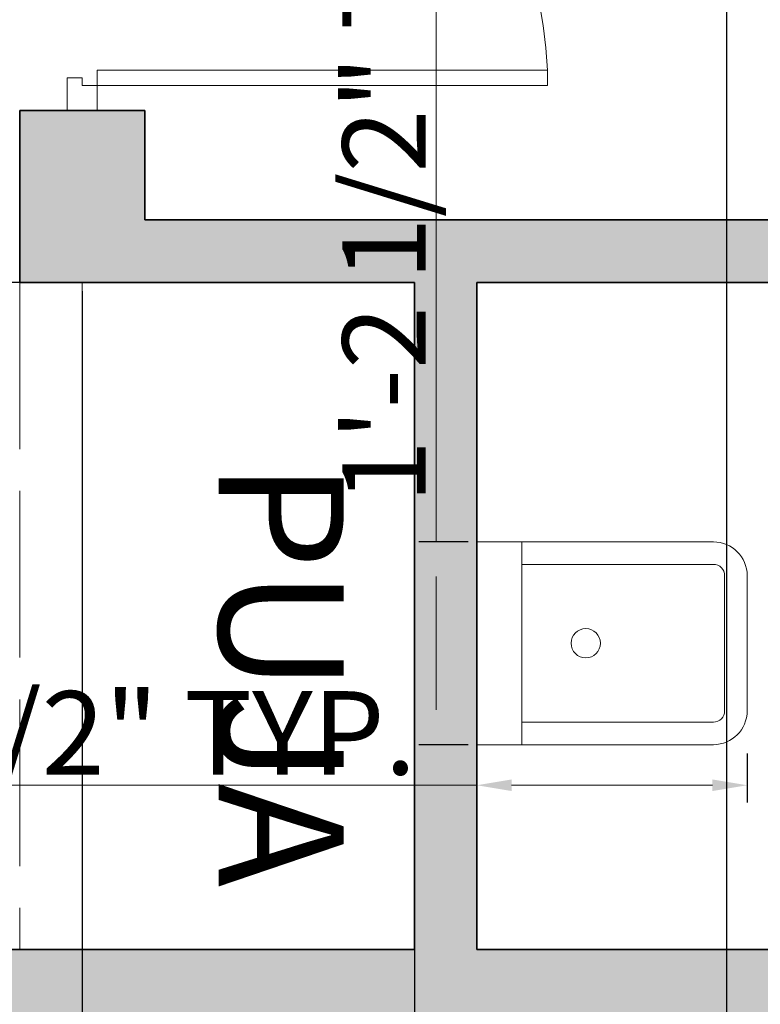
# Model space of a CAD drawing. Units: inches. Extents: x 2696 to 3240, y 1564 to 2310.
# Tile 66 of 76: x 3074 to 3127, y 2071 to 2142. Entities that reach past the tile are written whole.
import ezdxf

# ---------------------------------------------------------------- set-up
doc = ezdxf.new("R2010")
doc.units = ezdxf.units.IN
doc.linetypes.add('ACAD_ISO02W100', pattern=[15, 12, -3])
for name, color, linetype, lineweight in [('A-ANNO-DIMS', 3, 'Continuous', 18), ('A-AREA-IDEN', 7, 'Continuous', 18), ('A-DOOR', 4, 'Continuous', 18), ('A-FLOR-FIXT', 8, 'Continuous', 18), ('A-FURN', 251, 'Continuous', 13), ('A-WALL', 7, 'Continuous', 35), ('A-WALL-OVHD', 7, 'ACAD_ISO02W100', 18), ('A-WALL-PATT', 9, 'Continuous', 13)]:
    doc.layers.add(name, color=color, linetype=linetype, lineweight=lineweight)
doc.styles.add('TIMES NEW', font='times.ttf')
doc.styles.add('YQ_DIM', font='SUPEROS.SHX', dxfattribs={"width": 0.8, "bigfont": 'HZDX.SHX'})
doc.dimstyles.new('Siddhuu', dxfattribs={"dimtxt": 6, "dimasz": 2.5, "dimexe": 1.25, "dimexo": 0.625, "dimtad": 1, "dimdec": 1, "dimlunit": 4, "dimtxsty": 'TIMES NEW', "dimcen": 2.5, "dimclrd": 256, "dimclre": 1, "dimclrt": 7, "dimadec": 0, "dimazin": 0, "dimtfac": 1, "dimtdec": 1, "dimtmove": 0, "dimatfit": 3, "dimfxl": 1, "dimtolj": 1, "dimlwd": -1, "dimarcsym": 0})

# ---------------------------------------------------------------- blocks, each defined once
blk = doc.blocks.new('DR_D01')
for p, q in [((-0.45, 0.93), (-0.42, 0.93)), ((-0.45, 0.03), (-0.45, 0.93)), ((-0.42, 0.03), (-0.42, 0.93)), ((-0.5, 0.03), (-0.42, 0.03)), ((-0.5, 0.03), (-0.5, -0.03)), ((-0.45, 0.03), (-0.45, 0)), ((0.45, 0.03), (0.45, 0)), ((0.5, 0.03), (0.45, 0.03)), ((0.5, -0.03), (0.5, 0.03)), ((-0.45, 0), (-0.435, 0)), ((-0.435, 0), (-0.435, -0.03)), ((0.435, 0), (0.435, -0.03)), ((0.45, 0), (0.435, 0)), ((-0.435, -0.03), (-0.5, -0.03)), ((0.435, -0.03), (0.5, -0.03))]:
    blk.add_line(p, q)
blk.add_arc((-0.4602, 0.0206), 0.9103, 0.5915, 87.4664)
blk = doc.blocks.new('WC')
at = {"layer": 'A-FURN'}
for p, q in [((0, 14.59), (-17.022, 14.59)), ((-3.242, 14.59), (-3.242, 0)), ((-3.242, 12.969), (-17.022, 12.969)), ((-19.454, 2.432), (-19.454, 12.159)), ((-17.833, 2.432), (-17.833, 12.159)), ((-3.242, 1.621), (-17.022, 1.621)), ((0, 0), (-17.022, 0))]:
    blk.add_line(p, q, dxfattribs=at)
blk.add_circle((-7.836, 7.295), 1.051, dxfattribs=at)
for centre, radius, start, end in [((-17.022, 12.159), 2.432, 90, 180), ((-17.022, 12.159), 0.811, 90, 180), ((-17.022, 2.432), 2.432, 180, 270), ((-17.022, 2.432), 0.811, 180, 270)]:
    blk.add_arc(centre, radius, start, end, dxfattribs=at)
blk = doc.blocks.new('*D38')
at = {"layer": 'A-ANNO-DIMS', "color": 1, "lineweight": -2, "transparency": 16777216}
for p, q in [((3106.611, 2088.816), (3106.611, 2085.273)), ((3126.065, 2088.816), (3126.065, 2085.273))]:
    blk.add_line(p, q, dxfattribs=at)
at = {"layer": 'A-ANNO-DIMS', "transparency": 16777216}
for p, q in [((3106.611, 2086.523), (3035.395, 2086.523)), ((3123.565, 2086.523), (3109.111, 2086.523))]:
    blk.add_line(p, q, dxfattribs=at)
for points in [[(3109.111, 2086.94), (3109.111, 2086.107), (3106.611, 2086.523)], [(3123.565, 2086.94), (3123.565, 2086.107), (3126.065, 2086.523)]]:
    blk.add_solid(points, dxfattribs=at)
at = {"layer": 'Defpoints', "color": 0, "transparency": 16777216}
for p in [(3106.611, 2089.441), (3126.065, 2089.441), (3106.611, 2086.523)]:
    blk.add_point(p, dxfattribs=at)
at = {"layer": 'A-ANNO-DIMS', "color": 7, "transparency": 16777216, "insert": (3069.753, 2090.291), "char_height": 6, "attachment_point": 5, "style": 'TIMES NEW'}
blk.add_mtext('\\A1;WC 1\'-7 1/2" TYP.', dxfattribs=at)
blk = doc.blocks.new('*D39')
at = {"layer": 'A-ANNO-DIMS', "transparency": 16777216}
for p, q in [((3103.693, 2104.032), (3103.693, 2157.841)), ((3103.693, 2091.941), (3103.693, 2101.532))]:
    blk.add_line(p, q, dxfattribs=at)
at = {"layer": 'A-ANNO-DIMS', "color": 1, "lineweight": -2, "transparency": 16777216}
for p, q in [((3105.986, 2104.032), (3102.443, 2104.032)), ((3105.986, 2089.441), (3102.443, 2089.441))]:
    blk.add_line(p, q, dxfattribs=at)
at = {"layer": 'A-ANNO-DIMS', "transparency": 16777216}
for points in [[(3103.277, 2101.532), (3104.11, 2101.532), (3103.693, 2104.032)], [(3103.277, 2091.941), (3104.11, 2091.941), (3103.693, 2089.441)]]:
    blk.add_solid(points, dxfattribs=at)
at = {"layer": 'Defpoints', "color": 0, "transparency": 16777216}
for p in [(3103.693, 2104.032), (3106.611, 2104.032), (3106.611, 2089.441)]:
    blk.add_point(p, dxfattribs=at)
at = {"layer": 'A-ANNO-DIMS', "color": 7, "transparency": 16777216, "insert": (3099.932, 2132.186), "char_height": 6, "attachment_point": 5, "rotation": 90, "style": 'TIMES NEW'}
blk.add_mtext('\\A1;1\'-2 1/2" TYP.', dxfattribs=at)
blk = doc.blocks.new('*D54')
at = {"layer": 'A-ANNO-DIMS', "color": 1, "lineweight": -2, "transparency": 16777216}
for p, q in [((3124.611, 1893.826), (3124.611, 2298.451)), ((3136.611, 1893.826), (3136.611, 2298.451))]:
    blk.add_line(p, q, dxfattribs=at)
at = {"layer": 'A-ANNO-DIMS', "transparency": 16777216}
for p, q in [((3127.111, 2297.201), (3134.111, 2297.201)), ((3136.611, 2297.201), (3155.757, 2297.201))]:
    blk.add_line(p, q, dxfattribs=at)
for points in [[(3127.111, 2297.618), (3127.111, 2296.784), (3124.611, 2297.201)], [(3134.111, 2297.618), (3134.111, 2296.784), (3136.611, 2297.201)]]:
    blk.add_solid(points, dxfattribs=at)
at = {"layer": 'Defpoints', "color": 0, "transparency": 16777216}
for p in [(3136.611, 2297.201), (3124.611, 1893.201), (3136.611, 1893.201)]:
    blk.add_point(p, dxfattribs=at)
at = {"layer": 'A-ANNO-DIMS', "color": 7, "transparency": 16777216, "insert": (3147.434, 2300.878), "char_height": 6, "attachment_point": 5, "style": 'TIMES NEW'}
blk.add_mtext('\\A1;1\'-0"', dxfattribs=at)
blk = doc.blocks.new('*D65')
at = {"layer": 'A-ANNO-DIMS', "color": 1, "lineweight": -2, "transparency": 16777216}
for p, q in [((3078.209, 2122.076), (3078.209, 1568.951)), ((3102.111, 2122.076), (3102.111, 1568.951))]:
    blk.add_line(p, q, dxfattribs=at)
at = {"layer": 'A-ANNO-DIMS', "transparency": 16777216}
blk.add_line((3080.709, 1570.201), (3099.611, 1570.201), dxfattribs=at)
for points in [[(3080.709, 1570.618), (3080.709, 1569.784), (3078.209, 1570.201)], [(3099.611, 1570.618), (3099.611, 1569.784), (3102.111, 1570.201)]]:
    blk.add_solid(points, dxfattribs=at)
at = {"layer": 'Defpoints', "color": 0, "transparency": 16777216}
for p in [(3078.209, 2122.701), (3102.111, 2122.701), (3102.111, 1570.201)]:
    blk.add_point(p, dxfattribs=at)
at = {"layer": 'A-ANNO-DIMS', "color": 7, "transparency": 16777216, "insert": (3090.16, 1573.878), "char_height": 6, "attachment_point": 5, "style": 'TIMES NEW'}
blk.add_mtext('\\A1;2\'-0"', dxfattribs=at)
blk = doc.blocks.new('*D66')
at = {"layer": 'A-ANNO-DIMS', "color": 1, "lineweight": -2, "transparency": 16777216}
for p, q in [((3077.584, 2122.701), (2709.361, 2122.701)), ((3077.584, 2074.701), (2709.361, 2074.701))]:
    blk.add_line(p, q, dxfattribs=at)
at = {"layer": 'A-ANNO-DIMS', "transparency": 16777216}
blk.add_line((2710.611, 2077.201), (2710.611, 2120.201), dxfattribs=at)
for points in [[(2710.195, 2120.201), (2711.028, 2120.201), (2710.611, 2122.701)], [(2710.195, 2077.201), (2711.028, 2077.201), (2710.611, 2074.701)]]:
    blk.add_solid(points, dxfattribs=at)
at = {"layer": 'Defpoints', "color": 0, "transparency": 16777216}
for p in [(2710.611, 2122.701), (3078.209, 2122.701), (3078.209, 2074.701)]:
    blk.add_point(p, dxfattribs=at)
at = {"layer": 'A-ANNO-DIMS', "color": 7, "transparency": 16777216, "insert": (2706.934, 2098.701), "char_height": 6, "attachment_point": 5, "rotation": 90, "style": 'TIMES NEW'}
blk.add_mtext('\\A1;4\'-0"', dxfattribs=at)

msp = doc.modelspace()

# ---------------------------------------------------------------- hatches: boundary and pattern name
at = {"layer": 'A-WALL-PATT', "transparency": 33554556}
h = msp.add_hatch(color=256, dxfattribs=at)
h.dxf.hatch_style = 1
h.paths.add_polyline_path([(2879.111, 2253.201), (2905.91, 2253.201), (2905.91, 2262.201), (2841.889, 2262.201), (2841.889, 2253.201), (2870.111, 2253.201), (2870.111, 2176.601), (2965.709, 2176.601), (2965.709, 2206.701), (2973.583, 2206.701), (2973.583, 2215.701), (2965.709, 2215.701), (2965.709, 2262.201), (2929.91, 2262.201), (2929.91, 2253.201), (2956.709, 2253.201), (2956.709, 2185.601), (2879.111, 2185.601)])
h.paths.add_polyline_path([(2782.834, 2262.201), (2745.611, 2262.201), (2745.611, 2228.729), (2754.611, 2228.729), (2754.611, 2253.201), (2782.834, 2253.201)])
h.paths.add_polyline_path([(2754.611, 2136.201), (2965.709, 2136.201), (2965.709, 2145.201), (2879.111, 2145.201), (2879.111, 2147.074), (2877.34, 2147.074), (2870.111, 2147.074), (2870.111, 2145.201), (2754.611, 2145.201), (2754.611, 2169.674), (2745.611, 2169.674), (2745.611, 2000.201), (2754.611, 2000.201), (2754.611, 2019.201), (2849.083, 2019.201), (2849.083, 2023.701), (2841.209, 2023.701), (2841.209, 2051.827), (2836.709, 2051.827), (2836.709, 2023.701), (2754.611, 2023.701), (2754.611, 2091.201), (2836.709, 2091.201), (2836.709, 2087.827), (2841.209, 2087.827), (2841.209, 2095.701), (2754.611, 2095.701)])
h.paths.add_polyline_path([(2965.709, 2136.201), (2956.709, 2136.201), (2956.709, 2023.701), (2885.083, 2023.701), (2885.083, 2019.201), (2956.709, 2019.201), (2956.709, 1950.575), (2965.709, 1950.575), (2965.709, 1980.201), (2973.583, 1980.201), (2973.583, 1989.201), (2965.709, 1989.201)])
h.paths.add_polyline_path([(2754.611, 1906.701), (2880.209, 1906.701), (2884.709, 1906.701), (2956.709, 1906.701), (2956.709, 1792.701), (2944.709, 1792.701), (2944.709, 1783.701), (2956.709, 1783.701), (2956.709, 1740.201), (2884.709, 1740.201), (2884.709, 1783.701), (2896.709, 1783.701), (2896.709, 1792.701), (2884.709, 1792.701), (2884.709, 1846.701), (2880.209, 1846.701), (2880.209, 1740.201), (2754.611, 1740.201), (2754.611, 1777.201), (2745.611, 1777.201), (2745.611, 1692.701), (2754.611, 1692.701), (2754.611, 1731.201), (2956.709, 1731.201), (2956.709, 1723.327), (2965.709, 1723.327), (2965.709, 1884.201), (2973.583, 1884.201), (2973.583, 1893.201), (2965.709, 1893.201), (2965.709, 1914.575), (2956.709, 1914.575), (2956.709, 1911.201), (2754.611, 1911.201), (2754.611, 1930.201), (2745.611, 1930.201), (2745.611, 1817.201), (2754.611, 1817.201), (2754.611, 1854.201), (2826.611, 1854.201), (2826.611, 1868.827), (2822.111, 1868.827), (2822.111, 1858.701), (2754.611, 1858.701)])
h.paths.add_polyline_path([(2965.709, 1656.201), (3008.237, 1656.201), (3008.237, 1665.201), (2965.709, 1665.201), (2965.709, 1693.327), (2956.709, 1693.327), (2956.709, 1686.201), (2934.583, 1686.201), (2934.583, 1681.701), (2956.709, 1681.701), (2956.709, 1614.201), (2896.709, 1614.201), (2896.709, 1681.701), (2904.583, 1681.701), (2904.583, 1686.201), (2892.209, 1686.201), (2892.209, 1614.201), (2858.41, 1614.201), (2858.41, 1605.201), (2965.709, 1605.201)])
h.paths.add_polyline_path([(2788.41, 1614.201), (2754.611, 1614.201), (2754.611, 1652.701), (2745.611, 1652.701), (2745.611, 1605.201), (2788.41, 1605.201)])
h.paths.add_polyline_path([(3199.611, 1633.048), (3190.611, 1633.048), (3190.611, 1614.201), (3082.611, 1614.201), (3082.611, 1665.201), (3070.237, 1665.201), (3070.237, 1656.201), (3078.111, 1656.201), (3078.111, 1605.201), (3199.611, 1605.201)])
h.paths.add_polyline_path([(3199.611, 1702.048), (3190.611, 1702.048), (3190.611, 1699.701), (3106.611, 1699.701), (3106.611, 1747.701), (3190.611, 1747.701), (3190.611, 1752.201), (3082.611, 1752.201), (3082.611, 1760.075), (3078.111, 1760.075), (3078.111, 1747.701), (3102.111, 1747.701), (3102.111, 1699.701), (3078.111, 1699.701), (3078.111, 1695.201), (3190.611, 1695.201), (3190.611, 1676.355), (3199.611, 1676.355)])
h.paths.add_polyline_path([(3199.611, 1783.201), (3190.611, 1783.201), (3190.611, 1745.355), (3199.611, 1745.355)])
h.paths.add_polyline_path([(3082.611, 1884.201), (3190.611, 1884.201), (3190.611, 1853.201), (3199.611, 1853.201), (3199.611, 1901.701), (3190.611, 1901.701), (3190.611, 1893.201), (3005.583, 1893.201), (3005.583, 1891.281), (3005.583, 1884.201), (3078.111, 1884.201), (3078.111, 1792.075), (3082.611, 1792.075)])
h.paths.add_polyline_path([(3199.611, 1994.701), (3190.611, 1994.701), (3190.611, 1989.201), (3073.709, 1989.201), (3073.709, 2034.201), (3069.209, 2034.201), (3069.209, 1989.201), (3005.583, 1989.201), (3005.583, 1980.201), (3190.611, 1980.201), (3190.611, 1971.701), (3199.611, 1971.701)])
h.paths.add_polyline_path([(3199.611, 2155.201), (3190.611, 2155.201), (3190.611, 2064.701), (3199.611, 2064.701)])
h.paths.add_polyline_path([(3190.611, 2074.701), (3106.611, 2074.701), (3106.611, 2122.701), (3190.611, 2122.701), (3190.611, 2127.201), (3082.709, 2127.201), (3082.709, 2135.075), (3073.709, 2135.075), (3073.709, 2122.701), (3102.111, 2122.701), (3102.111, 2074.701), (3069.209, 2074.701), (3069.209, 2070.201), (3190.611, 2070.201)])
h.paths.add_polyline_path([(3082.709, 2253.201), (3190.611, 2253.201), (3190.611, 2225.201), (3199.611, 2225.201), (3199.611, 2262.201), (3073.709, 2262.201), (3073.709, 2215.701), (3035.583, 2215.701), (3035.583, 2206.701), (3073.709, 2206.701), (3073.709, 2171.075), (3082.709, 2171.075)])

# ---------------------------------------------------------------- linework, layer by layer
at = {"layer": 'A-WALL'}
for p, q in [((3082.709, 2135.075), (3073.709, 2135.075)), ((3073.709, 2135.075), (3073.709, 2122.701)), ((3082.709, 2127.201), (3082.709, 2135.075)), ((3082.709, 2127.201), (3190.611, 2127.201)), ((3073.709, 2122.701), (3102.111, 2122.701)), ((3102.111, 2074.701), (3102.111, 2122.701)), ((3106.611, 2122.701), (3190.611, 2122.701)), ((3106.611, 2074.701), (3106.611, 2122.701)), ((3069.209, 2074.701), (3102.111, 2074.701)), ((3106.611, 2074.701), (3190.611, 2074.701))]:
    msp.add_line(p, q, dxfattribs=at)
at = {"layer": 'A-WALL-OVHD'}
for p, q in [((3073.709, 2122.701), (3073.709, 2074.701)), ((3078.209, 2122.701), (3078.209, 2074.701))]:
    msp.add_line(p, q, dxfattribs=at)

# ---------------------------------------------------------------- block references
at = {"layer": 'A-DOOR', "xscale": 36, "yscale": -36, "zscale": 36, "rotation": 90}
msp.add_blockref('DR_D01', (3078.209, 2153.075), dxfattribs=at)
at = {"layer": 'A-FLOR-FIXT', "xscale": -1}
msp.add_blockref('WC', (3106.611, 2089.441), dxfattribs=at)

# ---------------------------------------------------------------- texts
at = {"layer": 'A-AREA-IDEN', "insert": (3097.035, 2109.85), "char_height": 9, "attachment_point": 1, "rotation": 270, "style": 'YQ_DIM'}
msp.add_mtext_dynamic_manual_height_columns('PUJA', width=48.00324, gutter_width=12.5, heights=[0], dxfattribs=at)

# ---------------------------------------------------------------- dimensions: what is measured, and where the dimension line sits
at = {"layer": 'A-ANNO-DIMS'}
for base, p1, p2, picture, middle in [((3136.611, 2297.201), (3124.611, 1893.201), (3136.611, 1893.201), '*D54', (3147.434, 2300.878)), ((3102.111, 1570.201), (3078.209, 2122.701), (3102.111, 2122.701), '*D65', (3090.16, 1573.878))]:
    dim = msp.add_linear_dim(base=base, p1=p1, p2=p2, dimstyle='Siddhuu', override={"dimdec": 1, "dimlfac": 1, "dimrnd": 0, "dimzin": 1, "dimdsep": 46, "dimlunit": 4, "dimfrac": 2}, dxfattribs=at)
    dim.commit()
    dim.dimension.update_dxf_attribs({"geometry": picture, "text_midpoint": middle})
for base, p1, p2, angle, text, picture, middle in [((3103.693, 2104.032), (3106.611, 2089.441), (3106.611, 2104.032), 90, '<> TYP.', '*D39', (3099.932, 2132.186)), ((3106.611, 2086.523), (3126.065, 2089.441), (3106.611, 2089.441), 180, 'WC <> TYP.', '*D38', (3069.753, 2090.291))]:
    dim = msp.add_linear_dim(base=base, p1=p1, p2=p2, angle=angle, text=text, dimstyle='Siddhuu', override={"dimdec": 1, "dimlfac": 1, "dimrnd": 0, "dimzin": 1, "dimdsep": 46, "dimlunit": 4, "dimfrac": 2}, dxfattribs=at)
    dim.commit()
    dim.dimension.update_dxf_attribs({"geometry": picture, "text_midpoint": middle})
dim = msp.add_linear_dim(base=(2710.611, 2122.701), p1=(3078.209, 2074.701), p2=(3078.209, 2122.701), angle=90, dimstyle='Siddhuu', override={"dimdec": 1, "dimlfac": 1, "dimrnd": 0, "dimzin": 1, "dimdsep": 46, "dimlunit": 4, "dimfrac": 2}, dxfattribs=at)
dim.commit()
dim.dimension.update_dxf_attribs({"geometry": '*D66', "text_midpoint": (2706.934, 2098.701)})

doc.saveas('drawing.dxf')
